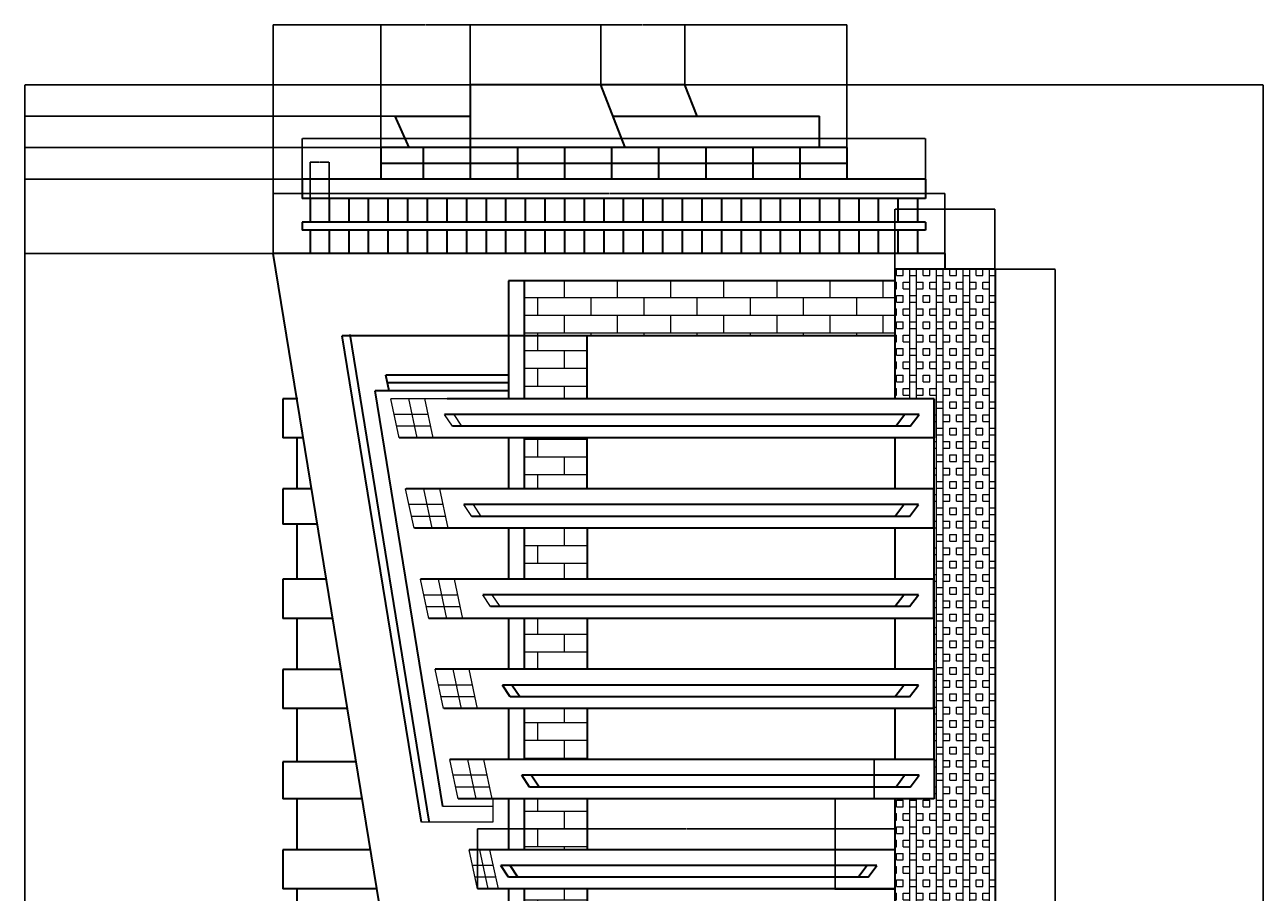
# Model space of a CAD drawing. Units: inches. Extents: x 597 to 2491, y 560 to 2558.
# Tile 2 of 2: x 597 to 2491, y 1231 to 2558. Entities that reach past the tile are written whole.
import ezdxf

# ---------------------------------------------------------------- set-up
doc = ezdxf.new("R2010")
doc.units = ezdxf.units.IN
for name, color, linetype, lineweight in [('A-ANNO-DIMS', 2, 'Continuous', 18), ('A-ELEV', 7, 'Continuous', 35), ('A-ELEV-PATT', 8, 'Continuous', 13), ('A-GLAZ', 4, 'Continuous', 18)]:
    doc.layers.add(name, color=color, linetype=linetype, lineweight=lineweight)
doc.styles.get("Standard").update_dxf_attribs({"font": 'arial.ttf'})
doc.dimstyles.get("Standard").update_dxf_attribs({"dimtxt": 0.18, "dimasz": 0.18, "dimexe": 0.18, "dimexo": 0.0625, "dimgap": 0.09, "dimtad": 0, "dimtih": 1, "dimtoh": 1, "dimdec": 4, "dimzin": 0, "dimdsep": 46, "dimtxsty": 'Standard', "dimcen": 0.09, "dimadec": 0, "dimazin": 0, "dimtfac": 1, "dimtdec": 4, "dimtofl": 0, "dimtmove": 0, "dimatfit": 3, "dimfxl": 1, "dimtolj": 1, "dimtzin": 0, "dimarcsym": 0})

# ---------------------------------------------------------------- blocks, each defined once
blk = doc.blocks.new('*D1')
at = {"layer": 'A-ANNO-DIMS', "color": 0, "lineweight": -2, "transparency": 16777216}
for p, q in [((1478.3, 2465.8), (2491, 2465.8)), ((2490.9, 2465.6), (2490.9, 1559)), ((2490.9, 652.1), (2490.9, 1558.7)), ((701.1, 651.9), (2491, 651.9))]:
    blk.add_line(p, q, dxfattribs=at)
at = {"layer": 'A-ANNO-DIMS', "color": 0, "transparency": 16777216}
for points in [[(2490.8, 2465.6), (2490.9, 2465.6), (2490.9, 2465.8)], [(2490.8, 652.1), (2490.9, 652.1), (2490.9, 651.9)]]:
    blk.add_solid(points, dxfattribs=at)
at = {"layer": 'Defpoints', "color": 0, "transparency": 16777216}
for p in [(1478.2, 2465.8), (2490.9, 2465.8), (701, 651.9)]:
    blk.add_point(p, dxfattribs=at)
at = {"layer": 'A-ANNO-DIMS', "color": 0, "transparency": 16777216, "insert": (2490.9, 1558.9), "char_height": 0.18, "attachment_point": 5}
blk.add_mtext('\\A1;1814', dxfattribs=at)
blk = doc.blocks.new('*D10')
at = {"layer": 'A-ANNO-DIMS', "color": 0, "lineweight": -2, "transparency": 16777216}
for p, q in [((976.9, 2207.9), (976.9, 2557.7)), ((977.1, 2557.6), (1058.8, 2557.6)), ((1141.3, 2557.6), (1059.7, 2557.6)), ((1141.5, 2369.9), (1141.5, 2557.7))]:
    blk.add_line(p, q, dxfattribs=at)
at = {"layer": 'A-ANNO-DIMS', "color": 0, "transparency": 16777216}
for points in [[(977.1, 2557.6), (977.1, 2557.5), (976.9, 2557.6)], [(1141.3, 2557.6), (1141.3, 2557.5), (1141.5, 2557.6)]]:
    blk.add_solid(points, dxfattribs=at)
at = {"layer": 'Defpoints', "color": 0, "transparency": 16777216}
for p in [(1141.5, 2557.6), (1141.5, 2369.8), (976.9, 2207.8)]:
    blk.add_point(p, dxfattribs=at)
at = {"layer": 'A-ANNO-DIMS', "color": 0, "transparency": 16777216, "insert": (1059.2, 2557.6), "char_height": 0.18, "attachment_point": 5}
blk.add_mtext('\\A1;164.54', dxfattribs=at)
blk = doc.blocks.new('*D11')
at = {"layer": 'A-ANNO-DIMS', "color": 0, "lineweight": -2, "transparency": 16777216}
for p, q in [((1141.5, 2369.9), (1141.5, 2557.7)), ((1141.7, 2557.6), (1209.5, 2557.6)), ((1278.3, 2557.6), (1210.4, 2557.6)), ((1278.4, 2465.9), (1278.4, 2557.7))]:
    blk.add_line(p, q, dxfattribs=at)
at = {"layer": 'A-ANNO-DIMS', "color": 0, "transparency": 16777216}
for points in [[(1141.7, 2557.6), (1141.7, 2557.5), (1141.5, 2557.6)], [(1278.3, 2557.6), (1278.3, 2557.5), (1278.4, 2557.6)]]:
    blk.add_solid(points, dxfattribs=at)
at = {"layer": 'Defpoints', "color": 0, "transparency": 16777216}
for p in [(1278.4, 2557.6), (1278.4, 2465.8), (1141.5, 2369.8)]:
    blk.add_point(p, dxfattribs=at)
at = {"layer": 'A-ANNO-DIMS', "color": 0, "transparency": 16777216, "insert": (1210, 2557.6), "char_height": 0.18, "attachment_point": 5}
blk.add_mtext('\\A1;136.96', dxfattribs=at)
blk = doc.blocks.new('*D12')
at = {"layer": 'A-ANNO-DIMS', "color": 0, "lineweight": -2, "transparency": 16777216}
for p, q in [((1278.4, 2465.9), (1278.4, 2557.7)), ((1278.6, 2557.6), (1378, 2557.6)), ((1478.1, 2557.6), (1378.7, 2557.6)), ((1478.2, 2465.9), (1478.2, 2557.7))]:
    blk.add_line(p, q, dxfattribs=at)
at = {"layer": 'A-ANNO-DIMS', "color": 0, "transparency": 16777216}
for points in [[(1278.6, 2557.6), (1278.6, 2557.5), (1278.4, 2557.6)], [(1478.1, 2557.6), (1478.1, 2557.5), (1478.2, 2557.6)]]:
    blk.add_solid(points, dxfattribs=at)
at = {"layer": 'Defpoints', "color": 0, "transparency": 16777216}
for p in [(1478.2, 2557.6), (1278.4, 2465.8), (1478.2, 2465.8)]:
    blk.add_point(p, dxfattribs=at)
at = {"layer": 'A-ANNO-DIMS', "color": 0, "transparency": 16777216, "insert": (1378.3, 2557.6), "char_height": 0.18, "attachment_point": 5}
blk.add_mtext('\\A1;199.8', dxfattribs=at)
blk = doc.blocks.new('*D13')
at = {"layer": 'A-ANNO-DIMS', "color": 0, "lineweight": -2, "transparency": 16777216}
for p, q in [((1478.2, 2465.9), (1478.2, 2557.7)), ((1478.4, 2557.6), (1542, 2557.6)), ((1606.6, 2557.6), (1542.9, 2557.6)), ((1606.7, 2465.9), (1606.7, 2557.7))]:
    blk.add_line(p, q, dxfattribs=at)
at = {"layer": 'A-ANNO-DIMS', "color": 0, "transparency": 16777216}
for points in [[(1478.4, 2557.6), (1478.4, 2557.5), (1478.2, 2557.6)], [(1606.6, 2557.6), (1606.6, 2557.5), (1606.7, 2557.6)]]:
    blk.add_solid(points, dxfattribs=at)
at = {"layer": 'Defpoints', "color": 0, "transparency": 16777216}
for p in [(1606.7, 2557.6), (1478.2, 2465.8), (1606.7, 2465.8)]:
    blk.add_point(p, dxfattribs=at)
at = {"layer": 'A-ANNO-DIMS', "color": 0, "transparency": 16777216, "insert": (1542.5, 2557.6), "char_height": 0.18, "attachment_point": 5}
blk.add_mtext('\\A1;128.52', dxfattribs=at)
blk = doc.blocks.new('*D14')
at = {"layer": 'A-ANNO-DIMS', "color": 0, "lineweight": -2, "transparency": 16777216}
for p, q in [((1606.7, 2465.9), (1606.7, 2557.7)), ((1606.9, 2557.6), (1730.2, 2557.6)), ((1854.3, 2557.6), (1731, 2557.6)), ((1854.4, 2369.9), (1854.4, 2557.7))]:
    blk.add_line(p, q, dxfattribs=at)
at = {"layer": 'A-ANNO-DIMS', "color": 0, "transparency": 16777216}
for points in [[(1606.9, 2557.6), (1606.9, 2557.5), (1606.7, 2557.6)], [(1854.3, 2557.6), (1854.3, 2557.5), (1854.4, 2557.6)]]:
    blk.add_solid(points, dxfattribs=at)
at = {"layer": 'Defpoints', "color": 0, "transparency": 16777216}
for p in [(1854.4, 2557.6), (1606.7, 2465.8), (1854.4, 2369.8)]:
    blk.add_point(p, dxfattribs=at)
at = {"layer": 'A-ANNO-DIMS', "color": 0, "transparency": 16777216, "insert": (1730.6, 2557.6), "char_height": 0.18, "attachment_point": 5}
blk.add_mtext('\\A1;247.7', dxfattribs=at)
blk = doc.blocks.new('*D19')
at = {"layer": 'A-ANNO-DIMS', "color": 0, "lineweight": -2, "transparency": 16777216}
for p, q in [((976.9, 2207.8), (597.1, 2207.8)), ((597.3, 2207.6), (597.3, 1656)), ((597.3, 1104), (597.3, 1655.6)), ((976.9, 1103.8), (597.1, 1103.8))]:
    blk.add_line(p, q, dxfattribs=at)
at = {"layer": 'A-ANNO-DIMS', "color": 0, "transparency": 16777216}
for points in [[(597.3, 2207.6), (597.3, 2207.6), (597.3, 2207.8)], [(597.3, 1104), (597.3, 1104), (597.3, 1103.8)]]:
    blk.add_solid(points, dxfattribs=at)
at = {"layer": 'Defpoints', "color": 0, "transparency": 16777216}
for p in [(597.3, 2207.8), (976.9, 2207.8), (976.9, 1103.8)]:
    blk.add_point(p, dxfattribs=at)
at = {"layer": 'A-ANNO-DIMS', "color": 0, "transparency": 16777216, "insert": (597.3, 1655.8), "char_height": 0.18, "attachment_point": 5}
blk.add_mtext('\\A1;1104', dxfattribs=at)
blk = doc.blocks.new('*D20')
at = {"layer": 'A-ANNO-DIMS', "color": 0, "lineweight": -2, "transparency": 16777216}
for p, q in [((1021.4, 2321.8), (597.1, 2321.8)), ((597.3, 2321.6), (597.3, 2265)), ((597.3, 2208), (597.3, 2264.6)), ((976.9, 2207.8), (597.1, 2207.8))]:
    blk.add_line(p, q, dxfattribs=at)
at = {"layer": 'A-ANNO-DIMS', "color": 0, "transparency": 16777216}
for points in [[(597.3, 2321.6), (597.3, 2321.6), (597.3, 2321.8)], [(597.3, 2208), (597.3, 2208), (597.3, 2207.8)]]:
    blk.add_solid(points, dxfattribs=at)
at = {"layer": 'Defpoints', "color": 0, "transparency": 16777216}
for p in [(597.3, 2321.8), (1021.5, 2321.8), (976.9, 2207.8)]:
    blk.add_point(p, dxfattribs=at)
at = {"layer": 'A-ANNO-DIMS', "color": 0, "transparency": 16777216, "insert": (597.3, 2264.8), "char_height": 0.18, "attachment_point": 5}
blk.add_mtext('\\A1;114', dxfattribs=at)
blk = doc.blocks.new('*D21')
at = {"layer": 'A-ANNO-DIMS', "color": 0, "lineweight": -2, "transparency": 16777216}
for p, q in [((1141.4, 2369.8), (597.1, 2369.8)), ((597.3, 2369.6), (597.3, 2346)), ((597.3, 2322), (597.3, 2345.6)), ((1141.4, 2321.8), (597.1, 2321.8))]:
    blk.add_line(p, q, dxfattribs=at)
at = {"layer": 'A-ANNO-DIMS', "color": 0, "transparency": 16777216}
for points in [[(597.3, 2369.6), (597.3, 2369.6), (597.3, 2369.8)], [(597.3, 2322), (597.3, 2322), (597.3, 2321.8)]]:
    blk.add_solid(points, dxfattribs=at)
at = {"layer": 'Defpoints', "color": 0, "transparency": 16777216}
for p in [(597.3, 2369.8), (1141.5, 2369.8), (1141.5, 2321.8)]:
    blk.add_point(p, dxfattribs=at)
at = {"layer": 'A-ANNO-DIMS', "color": 0, "transparency": 16777216, "insert": (597.3, 2345.8), "char_height": 0.18, "attachment_point": 5}
blk.add_mtext('\\A1;48', dxfattribs=at)
blk = doc.blocks.new('*D22')
at = {"layer": 'A-ANNO-DIMS', "color": 0, "lineweight": -2, "transparency": 16777216}
for p, q in [((1162.8, 2417.8), (597.1, 2417.8)), ((597.3, 2417.6), (597.3, 2394)), ((597.3, 2370), (597.3, 2393.6)), ((1141.4, 2369.8), (597.1, 2369.8))]:
    blk.add_line(p, q, dxfattribs=at)
at = {"layer": 'A-ANNO-DIMS', "color": 0, "transparency": 16777216}
for points in [[(597.3, 2417.6), (597.3, 2417.6), (597.3, 2417.8)], [(597.3, 2370), (597.3, 2370), (597.3, 2369.8)]]:
    blk.add_solid(points, dxfattribs=at)
at = {"layer": 'Defpoints', "color": 0, "transparency": 16777216}
for p in [(597.3, 2417.8), (1162.9, 2417.8), (1141.5, 2369.8)]:
    blk.add_point(p, dxfattribs=at)
at = {"layer": 'A-ANNO-DIMS', "color": 0, "transparency": 16777216, "insert": (597.3, 2393.8), "char_height": 0.18, "attachment_point": 5}
blk.add_mtext('\\A1;48', dxfattribs=at)
blk = doc.blocks.new('*D23')
at = {"layer": 'A-ANNO-DIMS', "color": 0, "lineweight": -2, "transparency": 16777216}
for p, q in [((1278.4, 2465.8), (597.1, 2465.8)), ((597.3, 2465.6), (597.3, 2442)), ((597.3, 2418), (597.3, 2441.6)), ((1162.8, 2417.8), (597.1, 2417.8))]:
    blk.add_line(p, q, dxfattribs=at)
at = {"layer": 'A-ANNO-DIMS', "color": 0, "transparency": 16777216}
for points in [[(597.3, 2465.6), (597.3, 2465.6), (597.3, 2465.8)], [(597.3, 2418), (597.3, 2418), (597.3, 2417.8)]]:
    blk.add_solid(points, dxfattribs=at)
at = {"layer": 'Defpoints', "color": 0, "transparency": 16777216}
for p in [(597.3, 2465.8), (1278.4, 2465.8), (1162.9, 2417.8)]:
    blk.add_point(p, dxfattribs=at)
at = {"layer": 'A-ANNO-DIMS', "color": 0, "transparency": 16777216, "insert": (597.3, 2441.8), "char_height": 0.18, "attachment_point": 5}
blk.add_mtext('\\A1;48', dxfattribs=at)
blk = doc.blocks.new('*D28')
at = {"layer": 'A-ANNO-DIMS', "color": 0, "lineweight": -2, "transparency": 16777216}
for p, q in [((1289.3, 1235.9), (1289.3, 1327.7)), ((1289.5, 1327.6), (1608.2, 1327.6)), ((1927.8, 1327.6), (1609, 1327.6)), ((1927.9, 1235.9), (1927.9, 1327.7))]:
    blk.add_line(p, q, dxfattribs=at)
at = {"layer": 'A-ANNO-DIMS', "color": 0, "transparency": 16777216}
for points in [[(1289.5, 1327.6), (1289.5, 1327.5), (1289.3, 1327.6)], [(1927.8, 1327.6), (1927.8, 1327.5), (1927.9, 1327.6)]]:
    blk.add_solid(points, dxfattribs=at)
at = {"layer": 'Defpoints', "color": 0, "transparency": 16777216}
for p in [(1927.9, 1327.6), (1289.3, 1235.8), (1927.9, 1235.8)]:
    blk.add_point(p, dxfattribs=at)
at = {"layer": 'A-ANNO-DIMS', "color": 0, "transparency": 16777216, "insert": (1608.6, 1327.6), "char_height": 0.18, "attachment_point": 5}
blk.add_mtext('\\A1;638.6', dxfattribs=at)
blk = doc.blocks.new('*D29')
at = {"layer": 'A-ANNO-DIMS', "color": 0, "lineweight": -2, "transparency": 16777216}
for p, q in [((1987.9, 1433.8), (1896, 1433.8)), ((1896.2, 1433.6), (1896.2, 1404)), ((1896.2, 1374), (1896.2, 1403.6)), ((1987.9, 1373.8), (1896, 1373.8))]:
    blk.add_line(p, q, dxfattribs=at)
at = {"layer": 'A-ANNO-DIMS', "color": 0, "transparency": 16777216}
for points in [[(1896.2, 1433.6), (1896.2, 1433.6), (1896.2, 1433.8)], [(1896.2, 1374), (1896.2, 1374), (1896.2, 1373.8)]]:
    blk.add_solid(points, dxfattribs=at)
at = {"layer": 'Defpoints', "color": 0, "transparency": 16777216}
for p in [(1896.2, 1433.8), (1987.9, 1433.8), (1987.9, 1373.8)]:
    blk.add_point(p, dxfattribs=at)
at = {"layer": 'A-ANNO-DIMS', "color": 0, "transparency": 16777216, "insert": (1896.2, 1403.8), "char_height": 0.18, "attachment_point": 5}
blk.add_mtext('\\A1;60', dxfattribs=at)
blk = doc.blocks.new('*D30')
at = {"layer": 'A-ANNO-DIMS', "color": 0, "lineweight": -2, "transparency": 16777216}
for p, q in [((1927.9, 1373.8), (1836, 1373.8)), ((1836.2, 1373.6), (1836.2, 1305)), ((1836.2, 1236), (1836.2, 1304.6)), ((1927.9, 1235.8), (1836, 1235.8))]:
    blk.add_line(p, q, dxfattribs=at)
at = {"layer": 'A-ANNO-DIMS', "color": 0, "transparency": 16777216}
for points in [[(1836.2, 1373.6), (1836.2, 1373.6), (1836.2, 1373.8)], [(1836.2, 1236), (1836.2, 1236), (1836.2, 1235.8)]]:
    blk.add_solid(points, dxfattribs=at)
at = {"layer": 'Defpoints', "color": 0, "transparency": 16777216}
for p in [(1836.2, 1373.8), (1927.9, 1373.8), (1927.9, 1235.8)]:
    blk.add_point(p, dxfattribs=at)
at = {"layer": 'A-ANNO-DIMS', "color": 0, "transparency": 16777216, "insert": (1836.2, 1304.8), "char_height": 0.18, "attachment_point": 5}
blk.add_mtext('\\A1;138', dxfattribs=at)
blk = doc.blocks.new('*D31')
at = {"layer": 'A-ANNO-DIMS', "color": 0, "lineweight": -2, "transparency": 16777216}
for p, q in [((1927.9, 2183.9), (1927.9, 2275.7)), ((1928.1, 2275.6), (2004.2, 2275.6)), ((2080.8, 2275.6), (2004.7, 2275.6)), ((2080.9, 2183.9), (2080.9, 2275.7))]:
    blk.add_line(p, q, dxfattribs=at)
at = {"layer": 'A-ANNO-DIMS', "color": 0, "transparency": 16777216}
for points in [[(1928.1, 2275.6), (1928.1, 2275.5), (1927.9, 2275.6)], [(2080.8, 2275.6), (2080.8, 2275.5), (2080.9, 2275.6)]]:
    blk.add_solid(points, dxfattribs=at)
at = {"layer": 'Defpoints', "color": 0, "transparency": 16777216}
for p in [(2080.9, 2275.6), (1927.9, 2183.8), (2080.9, 2183.8)]:
    blk.add_point(p, dxfattribs=at)
at = {"layer": 'A-ANNO-DIMS', "color": 0, "transparency": 16777216, "insert": (2004.4, 2275.6), "char_height": 0.18, "attachment_point": 5}
blk.add_mtext('\\A1;153', dxfattribs=at)
blk = doc.blocks.new('*D32')
at = {"layer": 'A-ANNO-DIMS', "color": 0, "lineweight": -2, "transparency": 16777216}
for p, q in [((2081, 2183.8), (2172.9, 2183.8)), ((2172.7, 2183.6), (2172.7, 1625.8)), ((2172.7, 1067.6), (2172.7, 1625.4)), ((2081, 1067.4), (2172.9, 1067.4))]:
    blk.add_line(p, q, dxfattribs=at)
at = {"layer": 'A-ANNO-DIMS', "color": 0, "transparency": 16777216}
for points in [[(2172.7, 2183.6), (2172.7, 2183.6), (2172.7, 2183.8)], [(2172.7, 1067.6), (2172.7, 1067.6), (2172.7, 1067.4)]]:
    blk.add_solid(points, dxfattribs=at)
at = {"layer": 'Defpoints', "color": 0, "transparency": 16777216}
for p in [(2080.9, 2183.8), (2080.9, 1067.4), (2172.7, 1067.4)]:
    blk.add_point(p, dxfattribs=at)
at = {"layer": 'A-ANNO-DIMS', "color": 0, "transparency": 16777216, "insert": (2172.7, 1625.6), "char_height": 0.18, "attachment_point": 5}
blk.add_mtext('\\A1;1116.4', dxfattribs=at)
blk = doc.blocks.new('*D33')
at = {"layer": 'A-ANNO-DIMS', "color": 0, "lineweight": -2, "transparency": 16777216}
for p, q in [((1021.5, 2291.9), (1021.5, 2383.7)), ((1021.7, 2383.6), (1497.7, 2383.6)), ((1974.3, 2383.6), (1498.3, 2383.6)), ((1974.4, 2291.9), (1974.4, 2383.7))]:
    blk.add_line(p, q, dxfattribs=at)
at = {"layer": 'A-ANNO-DIMS', "color": 0, "transparency": 16777216}
for points in [[(1021.7, 2383.6), (1021.7, 2383.5), (1021.5, 2383.6)], [(1974.3, 2383.6), (1974.3, 2383.5), (1974.4, 2383.6)]]:
    blk.add_solid(points, dxfattribs=at)
at = {"layer": 'Defpoints', "color": 0, "transparency": 16777216}
for p in [(1974.4, 2383.6), (1021.5, 2291.8), (1974.4, 2291.8)]:
    blk.add_point(p, dxfattribs=at)
at = {"layer": 'A-ANNO-DIMS', "color": 0, "transparency": 16777216, "insert": (1498, 2383.6), "char_height": 0.18, "attachment_point": 5}
blk.add_mtext('\\A1;953', dxfattribs=at)
blk = doc.blocks.new('*D34')
at = {"layer": 'A-ANNO-DIMS', "color": 0, "lineweight": -2, "transparency": 16777216}
for p, q in [((1033.5, 2255.9), (1033.5, 2347.7)), ((1033.7, 2347.6), (1047.5, 2347.6)), ((1062.3, 2347.6), (1048.4, 2347.6)), ((1062.4, 2255.9), (1062.4, 2347.7))]:
    blk.add_line(p, q, dxfattribs=at)
at = {"layer": 'A-ANNO-DIMS', "color": 0, "transparency": 16777216}
for points in [[(1033.7, 2347.6), (1033.7, 2347.5), (1033.5, 2347.6)], [(1062.3, 2347.6), (1062.3, 2347.5), (1062.4, 2347.6)]]:
    blk.add_solid(points, dxfattribs=at)
at = {"layer": 'Defpoints', "color": 0, "transparency": 16777216}
for p in [(1062.4, 2347.6), (1033.5, 2255.8), (1062.4, 2255.8)]:
    blk.add_point(p, dxfattribs=at)
at = {"layer": 'A-ANNO-DIMS', "color": 0, "transparency": 16777216, "insert": (1048, 2347.6), "char_height": 0.18, "attachment_point": 5}
blk.add_mtext('\\A1;28.957', dxfattribs=at)
blk = doc.blocks.new('*D35')
at = {"layer": 'A-ANNO-DIMS', "color": 0, "lineweight": -2, "transparency": 16777216}
for p, q in [((976.9, 2207.9), (976.9, 2299.7)), ((977.1, 2299.6), (1490.2, 2299.6)), ((2004.3, 2299.6), (1491.1, 2299.6)), ((2004.4, 2207.9), (2004.4, 2299.7))]:
    blk.add_line(p, q, dxfattribs=at)
at = {"layer": 'A-ANNO-DIMS', "color": 0, "transparency": 16777216}
for points in [[(977.1, 2299.6), (977.1, 2299.5), (976.9, 2299.6)], [(2004.3, 2299.6), (2004.3, 2299.5), (2004.4, 2299.6)]]:
    blk.add_solid(points, dxfattribs=at)
at = {"layer": 'Defpoints', "color": 0, "transparency": 16777216}
for p in [(2004.4, 2299.6), (976.9, 2207.8), (2004.4, 2207.8)]:
    blk.add_point(p, dxfattribs=at)
at = {"layer": 'A-ANNO-DIMS', "color": 0, "transparency": 16777216, "insert": (1490.7, 2299.6), "char_height": 0.18, "attachment_point": 5}
blk.add_mtext('\\A1;1027.5', dxfattribs=at)

msp = doc.modelspace()

# ---------------------------------------------------------------- hatches: boundary and pattern name
at = {"layer": 'A-ELEV-PATT'}
h = msp.add_hatch(dxfattribs=at)
h.set_pattern_fill('BOX', color=256, scale=1.6)
h.paths.add_polyline_path([(2080.9409, 2183.8154), (1987.9409, 2183.8154), (1987.9409, 1433.8154), (1987.9409, 1373.8154), (1927.9409, 1373.8154), (1927.9409, 1253.8154), (1927.9409, 1103.8154), (2080.9409, 1103.8154)])
h = msp.add_hatch(dxfattribs=at)
h.set_pattern_fill('BOX', color=256, scale=1.6)
h.paths.add_polyline_path([(2080.9409, 2183.8154), (1927.9409, 2183.8154), (1927.9409, 1985.8154), (1987.9409, 1985.8154), (2080.9409, 1985.8154)])
h = msp.add_hatch(dxfattribs=at)
h.set_pattern_fill('AR-BRSTD', color=256, scale=0.4)
h.paths.add_polyline_path([(1927.9409, 2165.8154), (1360.9409, 2165.8154), (1360.9409, 2081.8154), (1927.9409, 2081.8154)])
h.paths.add_polyline_path([(1456.9409, 2081.8154), (1360.9409, 2081.8154), (1360.9409, 1985.8154), (1456.9409, 1985.8154)])
h.paths.add_polyline_path([(1456.9409, 1925.8154), (1360.9409, 1925.8154), (1360.9409, 1847.8154), (1456.9409, 1847.8154)])
h.paths.add_polyline_path([(1456.9409, 1787.8154), (1360.9409, 1787.8154), (1360.9409, 1709.8154), (1456.9409, 1709.8154)])
h.paths.add_polyline_path([(1456.9409, 1649.8154), (1360.9409, 1649.8154), (1360.9409, 1571.8154), (1456.9409, 1571.8154)])
h.paths.add_polyline_path([(1456.9409, 1511.8154), (1360.9409, 1511.8154), (1360.9409, 1433.8154), (1456.9409, 1433.8154)])
h.paths.add_polyline_path([(1456.9409, 1373.8154), (1360.9409, 1373.8154), (1360.9409, 1295.8154), (1456.9409, 1295.8154)])
h.paths.add_polyline_path([(1456.9409, 1235.8154), (1360.9409, 1235.8154), (1360.9409, 1103.8154), (1456.9409, 1103.8154)])

# ---------------------------------------------------------------- linework, layer by layer
at = {"layer": 'A-ELEV'}
for p, q in [((1278.4409, 2465.8154), (1278.4409, 2321.8154)), ((1606.747, 2465.8154), (1278.4409, 2465.8154)), ((1515.0344, 2369.8154), (1478.2308, 2465.8154)), ((1625.1488, 2417.8154), (1606.747, 2465.8154)), ((1162.8521, 2417.8154), (1184.2199, 2369.8154)), ((1162.8521, 2417.8154), (1278.4409, 2417.8154)), ((1496.6326, 2417.8154), (1812.4648, 2417.8154)), ((1812.4648, 2369.8154), (1812.4648, 2417.8154)), ((1854.4409, 2369.8154), (1141.4843, 2369.8154)), ((1141.4843, 2369.8154), (1141.4843, 2321.8154)), ((1206.4409, 2369.8154), (1206.4409, 2321.8154)), ((1350.4409, 2369.8154), (1350.4409, 2321.8154)), ((1422.4409, 2369.8154), (1422.4409, 2321.8154)), ((1494.4409, 2369.8154), (1494.4409, 2321.8154)), ((1566.4409, 2369.8154), (1566.4409, 2321.8154)), ((1638.4409, 2369.8154), (1638.4409, 2321.8154)), ((1710.4409, 2369.8154), (1710.4409, 2321.8154)), ((1782.4409, 2369.8154), (1782.4409, 2321.8154)), ((1854.4409, 2369.8154), (1854.4409, 2321.8154)), ((1141.4843, 2345.8154), (1854.4409, 2345.8154)), ((1974.4409, 2321.8154), (1021.4843, 2321.8154)), ((1021.4843, 2321.8154), (1021.4843, 2291.8154)), ((1021.4843, 2321.8154), (1021.4843, 2306.8154)), ((1974.4409, 2321.8154), (1974.4409, 2291.8154)), ((1974.4409, 2291.8154), (1021.4843, 2291.8154)), ((1033.4843, 2291.8154), (1033.4843, 2255.8154)), ((1062.4409, 2291.8154), (1062.4409, 2255.8154)), ((1092.4409, 2291.8154), (1092.4409, 2255.8154)), ((1122.4409, 2291.8154), (1122.4409, 2255.8154)), ((1152.4409, 2291.8154), (1152.4409, 2255.8154)), ((1182.4409, 2291.8154), (1182.4409, 2255.8154)), ((1212.4409, 2291.8154), (1212.4409, 2255.8154)), ((1242.4409, 2291.8154), (1242.4409, 2255.8154)), ((1272.4409, 2291.8154), (1272.4409, 2255.8154)), ((1302.4409, 2291.8154), (1302.4409, 2255.8154)), ((1332.4409, 2291.8154), (1332.4409, 2255.8154)), ((1362.4409, 2291.8154), (1362.4409, 2255.8154)), ((1392.4409, 2291.8154), (1392.4409, 2255.8154)), ((1422.4409, 2291.8154), (1422.4409, 2255.8154)), ((1452.4409, 2291.8154), (1452.4409, 2255.8154)), ((1482.4409, 2291.8154), (1482.4409, 2255.8154)), ((1512.4409, 2291.8154), (1512.4409, 2255.8154)), ((1542.4409, 2291.8154), (1542.4409, 2255.8154)), ((1572.4409, 2291.8154), (1572.4409, 2255.8154)), ((1602.4409, 2291.8154), (1602.4409, 2255.8154)), ((1632.4409, 2291.8154), (1632.4409, 2255.8154)), ((1662.4409, 2291.8154), (1662.4409, 2255.8154)), ((1692.4409, 2291.8154), (1692.4409, 2255.8154)), ((1722.4409, 2291.8154), (1722.4409, 2255.8154)), ((1752.4409, 2291.8154), (1752.4409, 2255.8154)), ((1782.4409, 2291.8154), (1782.4409, 2255.8154)), ((1812.4409, 2291.8154), (1812.4409, 2255.8154)), ((1842.4409, 2291.8154), (1842.4409, 2255.8154)), ((1872.4409, 2291.8154), (1872.4409, 2255.8154)), ((1902.4409, 2291.8154), (1902.4409, 2255.8154)), ((1932.4409, 2291.8154), (1932.4409, 2255.8154)), ((1962.4409, 2291.8154), (1962.4409, 2255.8154)), ((1974.4409, 2255.8154), (1021.4843, 2255.8154)), ((1021.4843, 2255.8154), (1021.4843, 2243.8154)), ((1974.4409, 2255.8154), (1974.4409, 2243.8154)), ((1974.4409, 2243.8154), (1021.4843, 2243.8154)), ((1033.4843, 2243.8154), (1033.4843, 2207.8154)), ((1062.4409, 2243.8154), (1062.4409, 2207.8154)), ((1092.4409, 2243.8154), (1092.4409, 2207.8154)), ((1122.4409, 2243.8154), (1122.4409, 2207.8154)), ((1152.4409, 2243.8154), (1152.4409, 2207.8154)), ((1182.4409, 2243.8154), (1182.4409, 2207.8154)), ((1212.4409, 2243.8154), (1212.4409, 2207.8154)), ((1242.4409, 2243.8154), (1242.4409, 2207.8154)), ((1272.4409, 2243.8154), (1272.4409, 2207.8154)), ((1302.4409, 2243.8154), (1302.4409, 2207.8154)), ((1332.4409, 2243.8154), (1332.4409, 2207.8154)), ((1362.4409, 2243.8154), (1362.4409, 2207.8154)), ((1392.4409, 2243.8154), (1392.4409, 2207.8154)), ((1422.4409, 2243.8154), (1422.4409, 2207.8154)), ((1452.4409, 2243.8154), (1452.4409, 2207.8154)), ((1482.4409, 2243.8154), (1482.4409, 2207.8154)), ((1512.4409, 2243.8154), (1512.4409, 2207.8154)), ((1542.4409, 2243.8154), (1542.4409, 2207.8154)), ((1572.4409, 2243.8154), (1572.4409, 2207.8154)), ((1602.4409, 2243.8154), (1602.4409, 2207.8154)), ((1632.4409, 2243.8154), (1632.4409, 2207.8154)), ((1662.4409, 2243.8154), (1662.4409, 2207.8154)), ((1692.4409, 2243.8154), (1692.4409, 2207.8154)), ((1722.4409, 2243.8154), (1722.4409, 2207.8154)), ((1752.4409, 2243.8154), (1752.4409, 2207.8154)), ((1782.4409, 2243.8154), (1782.4409, 2207.8154)), ((1812.4409, 2243.8154), (1812.4409, 2207.8154)), ((1842.4409, 2243.8154), (1842.4409, 2207.8154)), ((1872.4409, 2243.8154), (1872.4409, 2207.8154)), ((1902.4409, 2243.8154), (1902.4409, 2207.8154)), ((1932.4409, 2243.8154), (1932.4409, 2207.8154)), ((1962.4409, 2243.8154), (1962.4409, 2207.8154)), ((2004.4409, 2207.8154), (976.9409, 2207.8154)), ((1156.9409, 1103.8154), (976.9409, 2207.8154)), ((2004.4409, 2183.8154), (2004.4409, 2207.8154)), ((1927.9409, 2183.8154), (1927.9409, 1985.8154)), ((2080.9409, 2183.8154), (1927.9409, 2183.8154)), ((2080.9409, 2183.8154), (2080.9409, 1103.8154)), ((1336.9409, 2165.8154), (1336.9409, 1985.8154)), ((1927.9409, 2165.8154), (1336.9409, 2165.8154)), ((1360.9409, 2165.8154), (1360.9409, 1985.8154)), ((1215.7415, 1339.7464), (1094.4371, 2083.7464)), ((1203.8979, 1337.8154), (1082.5935, 2081.8154)), ((1106.9104, 2081.8154), (1082.5935, 2081.8154)), ((1927.9409, 2081.8154), (1106.9104, 2081.8154)), ((1456.9409, 1985.8154), (1456.9409, 2081.8154)), ((1336.9409, 2021.8154), (1149.003, 2021.8154)), ((1154.1332, 1997.8154), (1149.003, 2021.8154)), ((1336.9409, 2009.8154), (1151.5681, 2009.8154)), ((1336.9409, 1997.8154), (1132.7645, 1997.8154)), ((1236.4602, 1361.8154), (1132.7645, 1997.8154)), ((1012.9409, 1985.8154), (991.8792, 1985.8154)), ((991.8792, 1985.8154), (991.8792, 1925.8154)), ((1012.9409, 1987.0154), (1012.9409, 1985.8154)), ((1987.9409, 1985.8154), (1243.0347, 1985.8154)), ((1987.9409, 1985.8154), (1987.9409, 1925.8154)), ((1987.9409, 1985.8154), (1987.9409, 1925.8154)), ((1987.9409, 1433.8154), (1987.9409, 1985.8154)), ((1964.7221, 1961.8154), (1239.2141, 1961.8154)), ((1928.998, 1943.8154), (1942.3253, 1961.8154)), ((1951.3948, 1943.8154), (1964.7221, 1961.8154)), ((1951.3948, 1943.8154), (1251.2076, 1943.8154)), ((1951.3948, 1943.8154), (1251.2076, 1943.8154)), ((1951.3948, 1943.8154), (1251.2076, 1943.8154)), ((1022.9191, 1925.8154), (991.8792, 1925.8154)), ((1012.9409, 1925.8154), (1012.9409, 1847.8154)), ((1987.9409, 1925.8154), (1169.5238, 1925.8154)), ((1336.9409, 1925.8154), (1336.9409, 1847.8154)), ((1360.9409, 1925.8154), (1360.9409, 1847.8154)), ((1456.9409, 1847.8154), (1456.9409, 1925.8154)), ((1927.9409, 1925.8154), (1927.9409, 1847.8154)), ((1035.6365, 1847.8154), (991.8792, 1847.8154)), ((991.8792, 1847.8154), (991.8792, 1794.074)), ((1986.8837, 1847.8154), (1180.3565, 1847.8154)), ((1986.8837, 1847.8154), (1986.8837, 1787.8154)), ((1963.6649, 1823.8154), (1268.6464, 1823.8154)), ((1927.9409, 1805.8154), (1941.2681, 1823.8154)), ((1950.3377, 1805.8154), (1963.6649, 1823.8154)), ((1950.3377, 1805.8154), (1280.64, 1805.8154)), ((1950.3377, 1805.8154), (1335.8837, 1805.8154)), ((1044.3987, 1794.074), (991.8792, 1794.074)), ((1012.9409, 1794.074), (1012.9409, 1709.8154)), ((1986.8837, 1787.8154), (1193.182, 1787.8154)), ((1336.9409, 1787.8154), (1336.9409, 1709.8154)), ((1360.9409, 1787.8154), (1360.9409, 1709.8154)), ((1456.9409, 1787.8154), (1456.9409, 1709.8154)), ((1927.9409, 1787.8154), (1927.9409, 1709.8154)), ((1058.1365, 1709.8154), (991.8792, 1709.8154)), ((991.8792, 1709.8154), (991.8792, 1649.8154)), ((1986.8837, 1709.8154), (1202.0043, 1709.8154)), ((1986.8837, 1709.8154), (1986.8837, 1649.8154)), ((1963.6649, 1685.8154), (1297.442, 1685.8154)), ((1927.9409, 1667.8154), (1941.2681, 1685.8154)), ((1950.3377, 1667.8154), (1963.6649, 1685.8154)), ((1950.3377, 1667.8154), (1309.4356, 1667.8154)), ((1950.3377, 1667.8154), (1309.4356, 1667.8154)), ((1067.9191, 1649.8154), (991.8792, 1649.8154)), ((1012.9409, 1649.8154), (1012.9409, 1571.7257)), ((1986.8837, 1649.8154), (1214.8298, 1649.8154)), ((1336.9409, 1649.8154), (1336.9409, 1571.8154)), ((1360.9409, 1649.8154), (1360.9409, 1571.8154)), ((1456.9409, 1649.8154), (1456.9409, 1571.8154)), ((1927.9409, 1649.8154), (1927.9409, 1571.8154)), ((1080.6512, 1571.7257), (991.8792, 1571.7257)), ((991.8792, 1571.7257), (991.8792, 1511.8154)), ((1986.8837, 1571.8154), (1224.5029, 1571.8154)), ((1986.8837, 1571.8154), (1986.8837, 1511.8154)), ((1963.6649, 1547.8154), (1327.6437, 1547.8154)), ((1339.6373, 1547.8154), (1327.6437, 1547.8154)), ((1339.6373, 1529.8154), (1327.6437, 1547.8154)), ((1354.0571, 1529.8154), (1342.0635, 1547.8154)), ((1927.9409, 1529.8154), (1941.2681, 1547.8154)), ((1950.3377, 1529.8154), (1963.6649, 1547.8154)), ((1950.3377, 1529.8154), (1339.6373, 1529.8154)), ((1950.3377, 1529.8154), (1339.6373, 1529.8154)), ((1950.3377, 1529.8154), (1339.6373, 1529.8154)), ((1090.4191, 1511.8154), (991.8792, 1511.8154)), ((1012.9409, 1511.8154), (1012.9409, 1430.3678)), ((1986.8837, 1511.8154), (1238.0062, 1511.8154)), ((1336.9409, 1511.8154), (1336.9409, 1433.8154)), ((1360.9409, 1511.8154), (1360.9409, 1433.8154)), ((1456.9409, 1511.8154), (1456.9409, 1433.8154)), ((1927.9409, 1511.8154), (1927.9409, 1433.8154)), ((1103.6986, 1430.3678), (991.8792, 1430.3678)), ((991.8792, 1430.3678), (991.8792, 1373.8154)), ((1987.9409, 1433.8154), (1247.0083, 1433.8154)), ((1987.9409, 1433.8154), (1987.9409, 1373.8154)), ((1369.1274, 1409.8551), (1357.1339, 1409.8551)), ((1369.1539, 1391.8154), (1357.1339, 1409.8551)), ((1964.7221, 1409.8154), (1357.1604, 1409.8154)), ((1383.5737, 1391.8154), (1371.5537, 1409.8551)), ((1928.998, 1391.8154), (1942.3253, 1409.8154)), ((1951.3948, 1391.8154), (1964.7221, 1409.8154)), ((1951.3948, 1391.8154), (1369.1539, 1391.8154)), ((1951.3948, 1391.8154), (1386.8134, 1391.8154)), ((1112.9191, 1373.8154), (991.8792, 1373.8154)), ((1012.9409, 1373.8154), (1012.9409, 1295.8154)), ((1987.9409, 1373.8154), (1259.8338, 1373.8154)), ((1336.9409, 1373.8154), (1336.9409, 1295.8154)), ((1360.9409, 1373.8154), (1360.9409, 1295.8154)), ((1456.9409, 1373.8154), (1456.9409, 1295.8154)), ((1927.9409, 1373.8154), (1927.9409, 1253.8154)), ((1125.6365, 1295.8154), (991.8792, 1295.8154)), ((991.8792, 1295.8154), (991.8792, 1235.8154)), ((1927.9409, 1295.8154), (1276.5069, 1295.8154)), ((1336.9409, 1253.8154), (1324.9474, 1271.8154)), ((1339.3672, 1271.8154), (1324.9474, 1271.8154)), ((1900.0554, 1271.8154), (1336.9409, 1271.8154)), ((1351.3607, 1253.8154), (1339.3672, 1271.8154)), ((1871.7969, 1253.8154), (1885.1242, 1271.8154)), ((1886.7281, 1253.8154), (1900.0554, 1271.8154)), ((1886.7281, 1253.8154), (1336.9409, 1253.8154)), ((1927.9409, 1253.8154), (1927.9409, 1103.8154)), ((1135.4191, 1235.8154), (991.8792, 1235.8154)), ((1012.9409, 1235.8154), (1012.9409, 1103.8154)), ((1927.9409, 1235.8154), (1289.3324, 1235.8154)), ((1336.9409, 1235.8154), (1336.9409, 1103.8154)), ((1360.9409, 1235.8154), (1360.9409, 1081.8154)), ((1456.9409, 1235.8154), (1456.9409, 1103.8154))]:
    msp.add_line(p, q, dxfattribs=at)
at = {"layer": 'A-GLAZ'}
for p, q in [((1169.5238, 1925.8154), (1156.6983, 1985.8154)), ((1243.0347, 1985.8154), (1156.6983, 1985.8154)), ((1197.1251, 1925.8558), (1184.2996, 1985.8558)), ((1221.6673, 1925.8558), (1208.8418, 1985.8558)), ((1213.972, 1961.8558), (1161.8198, 1961.8558)), ((1251.2076, 1961.8154), (1239.2141, 1961.8154)), ((1251.2076, 1943.8154), (1239.2141, 1961.8154)), ((1265.6275, 1943.8154), (1253.6339, 1961.8154)), ((1217.8196, 1943.8558), (1165.6675, 1943.8558)), ((1217.8196, 1943.8558), (1165.6675, 1943.8558)), ((1217.8196, 1943.8558), (1165.6675, 1943.8558)), ((1188.7099, 1847.7913), (1179.5066, 1847.7913)), ((1192.3557, 1787.6807), (1179.5302, 1847.6807)), ((1219.9421, 1787.7913), (1207.1166, 1847.7913)), ((1244.4842, 1787.7913), (1231.6587, 1847.7913)), ((1236.7889, 1823.7913), (1184.6368, 1823.7913)), ((1280.64, 1805.8154), (1268.6464, 1823.8154)), ((1290.3541, 1823.8154), (1278.3605, 1823.8154)), ((1295.0598, 1805.8154), (1283.0663, 1823.8154)), ((1240.6366, 1805.7913), (1188.4845, 1805.7913)), ((1240.6366, 1805.7913), (1188.4845, 1805.7913)), ((1240.6366, 1805.7913), (1188.4845, 1805.7913)), ((1214.8467, 1649.7364), (1202.0043, 1709.8154)), ((1242.563, 1649.2389), (1229.6142, 1709.8154)), ((1267.1052, 1649.2389), (1254.1564, 1709.8154)), ((1309.4356, 1685.8154), (1297.442, 1685.8154)), ((1309.4356, 1667.8154), (1297.442, 1685.8154)), ((1323.8554, 1667.8154), (1311.8619, 1685.8154)), ((1259.4099, 1685.2389), (1207.2577, 1685.2389)), ((1263.2575, 1667.2389), (1211.1054, 1667.2389)), ((1263.2575, 1667.2389), (1211.1054, 1667.2389)), ((1263.2575, 1667.2389), (1211.1054, 1667.2389)), ((1237.3512, 1511.7086), (1224.5029, 1571.8154)), ((1264.9803, 1511.6189), (1252.1128, 1571.8154)), ((1289.5225, 1511.6189), (1276.655, 1571.8154)), ((1281.8272, 1547.6189), (1229.6751, 1547.6189)), ((1285.6749, 1529.6189), (1233.5227, 1529.6189)), ((1285.6749, 1529.6189), (1233.5227, 1529.6189)), ((1285.6749, 1529.6189), (1233.5227, 1529.6189)), ((1256.2116, 1433.8154), (1247.0083, 1433.8154)), ((1259.8338, 1373.8154), (1247.0083, 1433.8154)), ((1287.4437, 1373.8154), (1274.6182, 1433.8154)), ((1311.9859, 1373.8154), (1299.1604, 1433.8154)), ((1304.2906, 1409.8154), (1252.1385, 1409.8154)), ((1308.1383, 1391.8154), (1255.9861, 1391.8154)), ((1308.1383, 1391.8154), (1255.9861, 1391.8154)), ((1312.9409, 1373.8154), (1312.9409, 1337.8154)), ((1312.9409, 1361.8154), (1236.4602, 1361.8154)), ((1312.9409, 1337.8154), (1203.8979, 1337.8154)), ((1289.3324, 1235.8154), (1276.5069, 1295.8154)), ((1305.9671, 1235.8154), (1293.1416, 1295.8154)), ((1321.306, 1235.8154), (1308.4805, 1295.8154)), ((1313.6107, 1271.8154), (1281.6371, 1271.8154)), ((1317.4583, 1253.8154), (1285.4848, 1253.8154))]:
    msp.add_line(p, q, dxfattribs=at)

# ---------------------------------------------------------------- dimensions: what is measured, and where the dimension line sits
at = {"layer": 'A-ANNO-DIMS'}
for base, p1, p2, override, picture, middle in [((1141.4843, 2557.5654), (976.9409, 2207.8154), (1141.4843, 2369.8154), {"dimdec": 2, "dimlfac": 1, "dimrnd": 0, "dimzin": 0, "dimdsep": 46, "dimlunit": 2}, '*D10', (1059.2126, 2557.5654)), ((1278.4409, 2557.5654), (1141.4843, 2369.8154), (1278.4409, 2465.8154), {"dimdec": 2, "dimlfac": 1, "dimrnd": 0, "dimzin": 0, "dimdsep": 46, "dimlunit": 2}, '*D11', (1209.9626, 2557.5654)), ((1478.2308, 2557.5654), (1278.4409, 2465.8154), (1478.2308, 2465.8154), {"dimdec": 1, "dimlfac": 1, "dimrnd": 0, "dimzin": 0, "dimdsep": 46, "dimlunit": 2}, '*D12', (1378.3358, 2557.5654)), ((1606.747, 2557.5654), (1478.2308, 2465.8154), (1606.747, 2465.8154), {"dimdec": 2, "dimlfac": 1, "dimrnd": 0, "dimzin": 0, "dimdsep": 46, "dimlunit": 2}, '*D13', (1542.4889, 2557.5654)), ((1854.4409, 2557.5654), (1606.747, 2465.8154), (1854.4409, 2369.8154), {"dimdec": 1, "dimlfac": 1, "dimrnd": 0, "dimzin": 0, "dimdsep": 46, "dimlunit": 2}, '*D14', (1730.5939, 2557.5654)), ((1974.4409, 2383.5654), (1021.4843, 2291.8154), (1974.4409, 2291.8154), {"dimdec": 0, "dimlfac": 1, "dimrnd": 0, "dimzin": 0, "dimdsep": 46, "dimlunit": 2}, '*D33', (1497.9626, 2383.5654)), ((1062.4409, 2347.5654), (1033.4843, 2255.8154), (1062.4409, 2255.8154), {"dimdec": 3, "dimlfac": 1, "dimrnd": 0, "dimzin": 0, "dimdsep": 46, "dimlunit": 2}, '*D34', (1047.9626, 2347.5654)), ((2004.4409, 2299.5654), (976.9409, 2207.8154), (2004.4409, 2207.8154), {"dimdec": 1, "dimlfac": 1, "dimrnd": 0, "dimzin": 0, "dimdsep": 46, "dimlunit": 2}, '*D35', (1490.6909, 2299.5654)), ((1927.9409, 1327.5654), (1289.3324, 1235.8154), (1927.9409, 1235.8154), {"dimdec": 1, "dimlfac": 1, "dimrnd": 0, "dimzin": 0, "dimdsep": 46, "dimlunit": 2}, '*D28', (1608.6367, 1327.5654))]:
    dim = msp.add_linear_dim(base=base, p1=p1, p2=p2, dimstyle='Standard', override=override, dxfattribs=at)
    dim.commit()
    dim.dimension.update_dxf_attribs({"geometry": picture, "text_midpoint": middle})
for base, p1, p2, angle, override, picture, middle in [((597.2924, 2465.8154), (1162.8521, 2417.8154), (1278.4409, 2465.8154), 90, {"dimdec": 0, "dimlfac": 1, "dimrnd": 0, "dimzin": 0, "dimdsep": 46, "dimlunit": 2}, '*D23', (597.2924, 2441.8154)), ((2490.8684, 2465.8154), (701.0424, 651.9147), (1478.2308, 2465.8154), 90, {"dimdec": 0, "dimlfac": 1, "dimrnd": 0, "dimzin": 0, "dimdsep": 46, "dimlunit": 2}, '*D1', (2490.8684, 1558.865)), ((597.2924, 2417.8154), (1141.4843, 2369.8154), (1162.8521, 2417.8154), 90, {"dimdec": 0, "dimlfac": 1, "dimrnd": 0, "dimzin": 0, "dimdsep": 46, "dimlunit": 2}, '*D22', (597.2924, 2393.8154)), ((597.2924, 2369.8154), (1141.4843, 2321.8154), (1141.4843, 2369.8154), 90, {"dimdec": 0, "dimlfac": 1, "dimrnd": 0, "dimzin": 0, "dimdsep": 46, "dimlunit": 2}, '*D21', (597.2924, 2345.8154)), ((597.2924, 2321.8154), (976.9409, 2207.8154), (1021.4843, 2321.8154), 90, {"dimdec": 0, "dimlfac": 1, "dimrnd": 0, "dimzin": 0, "dimdsep": 46, "dimlunit": 2}, '*D20', (597.2924, 2264.8154)), ((2080.9409, 2275.5654), (1927.9409, 2183.8154), (2080.9409, 2183.8154), 0, {"dimdec": 0, "dimlfac": 1, "dimrnd": 0, "dimzin": 0, "dimdsep": 46, "dimlunit": 2}, '*D31', (2004.4409, 2275.5654)), ((597.2924, 2207.8154), (976.9409, 1103.8154), (976.9409, 2207.8154), 90, {"dimdec": 0, "dimlfac": 1, "dimrnd": 0, "dimzin": 0, "dimdsep": 46, "dimlunit": 2}, '*D19', (597.2924, 1655.8154)), ((2172.6909, 1067.4311), (2080.9409, 2183.8154), (2080.9409, 1067.4311), 270, {"dimdec": 1, "dimlfac": 1, "dimrnd": 0, "dimzin": 0, "dimdsep": 46, "dimlunit": 2}, '*D32', (2172.6909, 1625.6232)), ((1896.1909, 1433.8154), (1987.9409, 1373.8154), (1987.9409, 1433.8154), 90, {"dimdec": 0, "dimlfac": 1, "dimrnd": 0, "dimzin": 0, "dimdsep": 46, "dimlunit": 2}, '*D29', (1896.1909, 1403.8154)), ((1836.1909, 1373.8154), (1927.9409, 1235.8154), (1927.9409, 1373.8154), 90, {"dimdec": 0, "dimlfac": 1, "dimrnd": 0, "dimzin": 0, "dimdsep": 46, "dimlunit": 2}, '*D30', (1836.1909, 1304.8154))]:
    dim = msp.add_linear_dim(base=base, p1=p1, p2=p2, angle=angle, dimstyle='Standard', override=override, dxfattribs=at)
    dim.commit()
    dim.dimension.update_dxf_attribs({"geometry": picture, "text_midpoint": middle})

doc.saveas('drawing.dxf')
